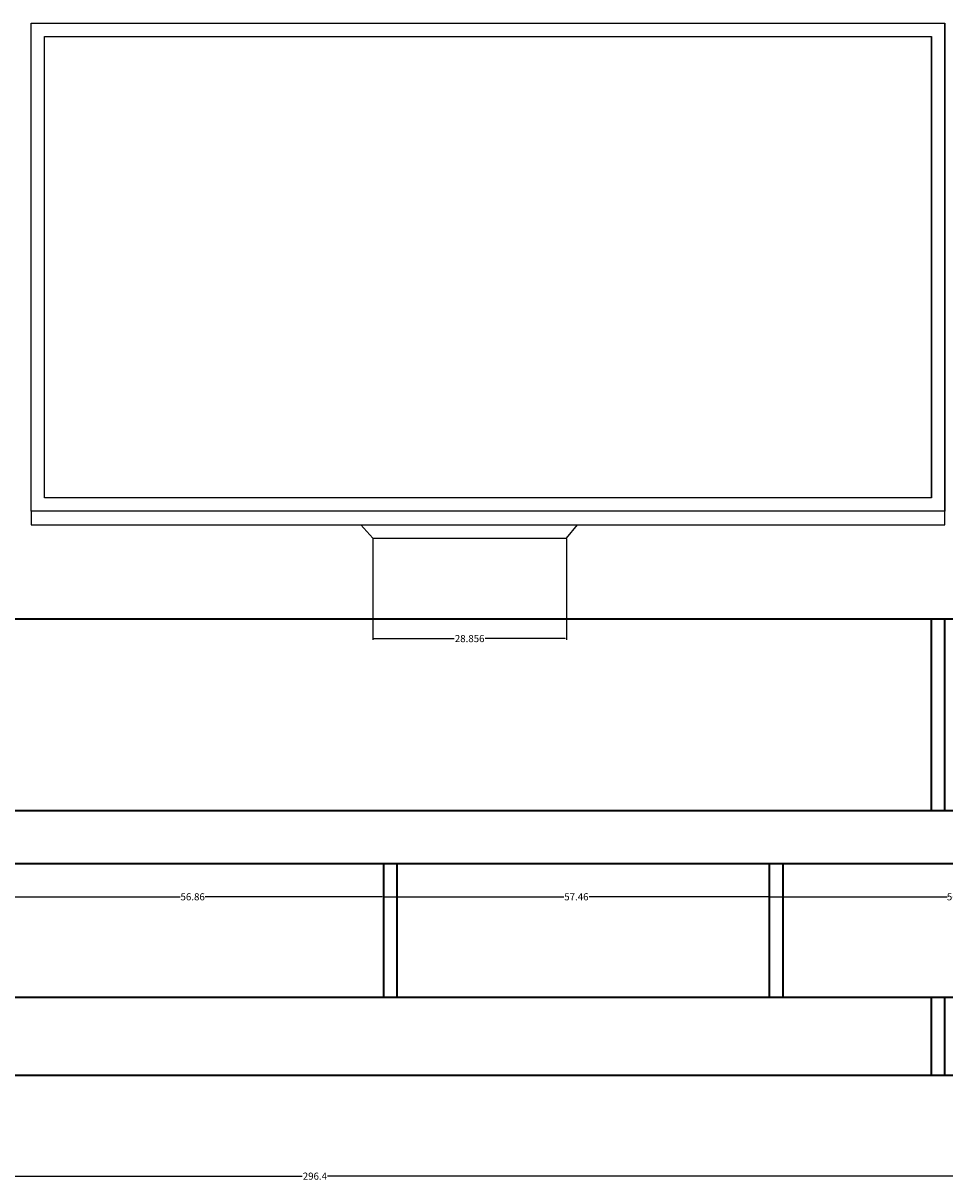
# Model space of a CAD drawing. Units: inches. Extents: x 35 to 365, y 67 to 380.
# Tile 3 of 5: x 156 to 293, y 67 to 240. Entities that reach past the tile are written whole.
import ezdxf

# ---------------------------------------------------------------- set-up
doc = ezdxf.new("R2010")
doc.units = ezdxf.units.IN
doc.header["$MEASUREMENT"] = 0
for name, color, linetype, lineweight in [('A-ANNO-DIMS', 2, 'Continuous', 18), ('A-EQPM', 4, 'Continuous', 25), ('A-FURN', 7, 'Continuous', 35)]:
    doc.layers.add(name, color=color, linetype=linetype, lineweight=lineweight)
doc.styles.get("Standard").update_dxf_attribs({"font": 'arial.ttf'})
doc.dimstyles.get("Standard").update_dxf_attribs({"dimtxt": 1.0625, "dimasz": 0.18, "dimexe": 0.18, "dimexo": 0.0625, "dimgap": 0.09, "dimtad": 0, "dimtih": 1, "dimtoh": 1, "dimdec": 4, "dimzin": 0, "dimdsep": 46, "dimlunit": 4, "dimtxsty": 'Standard', "dimcen": 0.09, "dimadec": 0, "dimazin": 0, "dimtfac": 1, "dimtdec": 4, "dimtofl": 0, "dimtmove": 0, "dimatfit": 3, "dimfxl": 1, "dimtolj": 1, "dimtzin": 0, "dimarcsym": 0})

# ---------------------------------------------------------------- blocks, each defined once
blk = doc.blocks.new('*D9')
at = {"layer": 'A-ANNO-DIMS', "color": 0, "lineweight": -2, "transparency": 16777216}
for p, q in [((51.28, 94.63), (51.28, 67.85)), ((347.67, 82.99), (347.67, 67.85)), ((51.46, 68.03), (197.58, 68.03)), ((347.49, 68.03), (201.36, 68.03))]:
    blk.add_line(p, q, dxfattribs=at)
at = {"layer": 'A-ANNO-DIMS', "color": 0, "transparency": 16777216}
for points in [[(51.46, 68.06), (51.46, 68), (51.28, 68.03)], [(347.49, 68.06), (347.49, 68), (347.67, 68.03)]]:
    blk.add_solid(points, dxfattribs=at)
at = {"layer": 'Defpoints', "color": 0, "transparency": 16777216}
for p in [(51.28, 94.7), (347.67, 83.05), (347.67, 68.03)]:
    blk.add_point(p, dxfattribs=at)
at = {"layer": 'A-ANNO-DIMS', "color": 0, "transparency": 16777216, "insert": (199.47, 68.03), "char_height": 1.062, "attachment_point": 5}
blk.add_mtext('\\A1;296.4', dxfattribs=at)
blk = doc.blocks.new('*D18')
at = {"layer": 'A-ANNO-DIMS', "color": 0, "lineweight": -2, "transparency": 16777216}
for p, q in [((152.83, 94.76), (152.83, 109.83)), ((153.01, 109.65), (179.38, 109.65)), ((209.51, 109.65), (183.14, 109.65)), ((209.69, 94.76), (209.69, 109.83))]:
    blk.add_line(p, q, dxfattribs=at)
at = {"layer": 'A-ANNO-DIMS', "color": 0, "transparency": 16777216}
for points in [[(153.01, 109.68), (153.01, 109.62), (152.83, 109.65)], [(209.51, 109.68), (209.51, 109.62), (209.69, 109.65)]]:
    blk.add_solid(points, dxfattribs=at)
at = {"layer": 'Defpoints', "color": 0, "transparency": 16777216}
for p in [(209.69, 109.65), (152.83, 94.7), (209.69, 94.7)]:
    blk.add_point(p, dxfattribs=at)
at = {"layer": 'A-ANNO-DIMS', "color": 0, "transparency": 16777216, "insert": (181.26, 109.65), "char_height": 1.062, "attachment_point": 5}
blk.add_mtext('\\A1;56.86', dxfattribs=at)
blk = doc.blocks.new('*D19')
at = {"layer": 'A-ANNO-DIMS', "color": 0, "lineweight": -2, "transparency": 16777216}
for p, q in [((209.69, 94.76), (209.69, 109.83)), ((209.87, 109.65), (236.54, 109.65)), ((266.98, 109.65), (240.31, 109.65)), ((267.16, 94.76), (267.16, 109.83))]:
    blk.add_line(p, q, dxfattribs=at)
at = {"layer": 'A-ANNO-DIMS', "color": 0, "transparency": 16777216}
for points in [[(209.87, 109.68), (209.87, 109.62), (209.69, 109.65)], [(266.98, 109.68), (266.98, 109.62), (267.16, 109.65)]]:
    blk.add_solid(points, dxfattribs=at)
at = {"layer": 'Defpoints', "color": 0, "transparency": 16777216}
for p in [(267.16, 109.65), (209.69, 94.7), (267.16, 94.7)]:
    blk.add_point(p, dxfattribs=at)
at = {"layer": 'A-ANNO-DIMS', "color": 0, "transparency": 16777216, "insert": (238.42, 109.65), "char_height": 1.062, "attachment_point": 5}
blk.add_mtext('\\A1;57.46', dxfattribs=at)
blk = doc.blocks.new('*D20')
at = {"layer": 'A-ANNO-DIMS', "color": 0, "lineweight": -2, "transparency": 16777216}
for p, q in [((267.16, 94.76), (267.16, 109.83)), ((267.34, 109.65), (293.63, 109.65)), ((323.49, 109.65), (297.19, 109.65)), ((323.67, 94.76), (323.67, 109.83))]:
    blk.add_line(p, q, dxfattribs=at)
at = {"layer": 'A-ANNO-DIMS', "color": 0, "transparency": 16777216}
for points in [[(267.34, 109.68), (267.34, 109.62), (267.16, 109.65)], [(323.49, 109.68), (323.49, 109.62), (323.67, 109.65)]]:
    blk.add_solid(points, dxfattribs=at)
at = {"layer": 'Defpoints', "color": 0, "transparency": 16777216}
for p in [(323.67, 109.65), (267.16, 94.7), (323.67, 94.7)]:
    blk.add_point(p, dxfattribs=at)
at = {"layer": 'A-ANNO-DIMS', "color": 0, "transparency": 16777216, "insert": (295.41, 109.65), "char_height": 1.062, "attachment_point": 5}
blk.add_mtext('\\A1;56.51', dxfattribs=at)
blk = doc.blocks.new('*D31')
at = {"layer": 'A-ANNO-DIMS', "color": 0, "lineweight": -2, "transparency": 16777216}
for p, q in [((208.09, 163), (208.09, 147.94)), ((236.95, 163), (236.95, 147.94)), ((208.27, 148.12), (220.22, 148.12)), ((236.77, 148.12), (224.82, 148.12))]:
    blk.add_line(p, q, dxfattribs=at)
at = {"layer": 'A-ANNO-DIMS', "color": 0, "transparency": 16777216}
for points in [[(208.27, 148.15), (208.27, 148.09), (208.09, 148.12)], [(236.77, 148.15), (236.77, 148.09), (236.95, 148.12)]]:
    blk.add_solid(points, dxfattribs=at)
at = {"layer": 'Defpoints', "color": 0, "transparency": 16777216}
for p in [(208.09, 163.07), (236.95, 163.07), (208.09, 148.12)]:
    blk.add_point(p, dxfattribs=at)
at = {"layer": 'A-ANNO-DIMS', "color": 0, "transparency": 16777216, "insert": (222.52, 148.12), "char_height": 1.062, "attachment_point": 5}
blk.add_mtext('\\A1;28.856', dxfattribs=at)

msp = doc.modelspace()

# ---------------------------------------------------------------- linework, layer by layer
at = {"layer": 'A-EQPM'}
for p, q in [((293.3029, 165.0829), (293.3029, 239.8076)), ((291.3029, 169.0829), (291.3029, 237.8076)), ((157.1904, 167.0829), (157.1904, 165.0829)), ((293.3029, 165.0829), (293.3029, 167.0829)), ((157.1904, 165.0829), (293.3029, 165.0829)), ((206.2863, 165.0829), (208.0914, 163.0669)), ((236.9477, 163.0669), (238.5912, 165.0829)), ((208.0914, 163.0669), (236.9477, 163.0669))]:
    msp.add_line(p, q, dxfattribs=at)
for points in [[(157.1904, 239.8076), (293.3029, 239.8076), (293.3029, 167.0829), (157.1904, 167.0829)], [(159.1904, 237.8076), (291.3029, 237.8076), (291.3029, 169.0829), (159.1904, 169.0829)]]:
    msp.add_lwpolyline(points, close=True, dxfattribs=at)
at = {"layer": 'A-FURN'}
for p, q in [((291.3029, 122.4805), (291.3029, 151.0198)), ((293.3029, 122.4805), (293.3029, 151.0198)), ((323.6655, 122.4805), (115.383, 122.4805)), ((323.6655, 114.5646), (51.2797, 114.5646)), ((209.6918, 114.5646), (209.6918, 94.6954)), ((211.6918, 114.5646), (211.6918, 94.6954)), ((267.1558, 114.5646), (267.1558, 94.6954)), ((269.1558, 114.5646), (269.1558, 94.6954)), ((51.2797, 94.6954), (323.6655, 94.6954)), ((291.3029, 82.9768), (291.3029, 94.6954)), ((293.3029, 82.9768), (293.3029, 94.6954)), ((61.3227, 83.0529), (347.6655, 83.0529))]:
    msp.add_line(p, q, dxfattribs=at)
msp.add_lwpolyline([(115.383, 254.0695), (323.6655, 254.0695), (323.6655, 151.0198), (115.383, 151.0198)], close=True, dxfattribs=at)

# ---------------------------------------------------------------- dimensions: what is measured, and where the dimension line sits
at = {"layer": 'A-ANNO-DIMS'}
for base, p1, p2, angle, override, picture, middle in [((208.0914, 148.1169), (236.9477, 163.0669), (208.0914, 163.0669), 180, {"dimdec": 3, "dimlfac": 1, "dimrnd": 0, "dimzin": 0, "dimdsep": 46, "dimlunit": 2}, '*D31', (222.5195, 148.1169)), ((209.6918, 109.6454), (152.8319, 94.6954), (209.6918, 94.6954), 0, {"dimdec": 2, "dimlfac": 1, "dimrnd": 0, "dimzin": 0, "dimdsep": 46, "dimlunit": 2}, '*D18', (181.2619, 109.6454))]:
    dim = msp.add_linear_dim(base=base, p1=p1, p2=p2, angle=angle, dimstyle='Standard', override=override, dxfattribs=at)
    dim.commit()
    dim.dimension.update_dxf_attribs({"geometry": picture, "text_midpoint": middle})
for base, p1, p2, override, picture, middle in [((267.1558, 109.6454), (209.6918, 94.6954), (267.1558, 94.6954), {"dimdec": 2, "dimlfac": 1, "dimrnd": 0, "dimzin": 0, "dimdsep": 46, "dimlunit": 2}, '*D19', (238.4238, 109.6454)), ((323.6655, 109.6454), (267.1558, 94.6954), (323.6655, 94.6954), {"dimdec": 2, "dimlfac": 1, "dimrnd": 0, "dimzin": 0, "dimdsep": 46, "dimlunit": 2}, '*D20', (295.4107, 109.6454)), ((347.6655, 68.0268), (51.2797, 94.6954), (347.6655, 83.0529), {"dimdec": 1, "dimlfac": 1, "dimrnd": 0, "dimzin": 0, "dimdsep": 46, "dimlunit": 2}, '*D9', (199.4726, 68.0268))]:
    dim = msp.add_linear_dim(base=base, p1=p1, p2=p2, dimstyle='Standard', override=override, dxfattribs=at)
    dim.commit()
    dim.dimension.update_dxf_attribs({"geometry": picture, "text_midpoint": middle})

doc.saveas('drawing.dxf')
